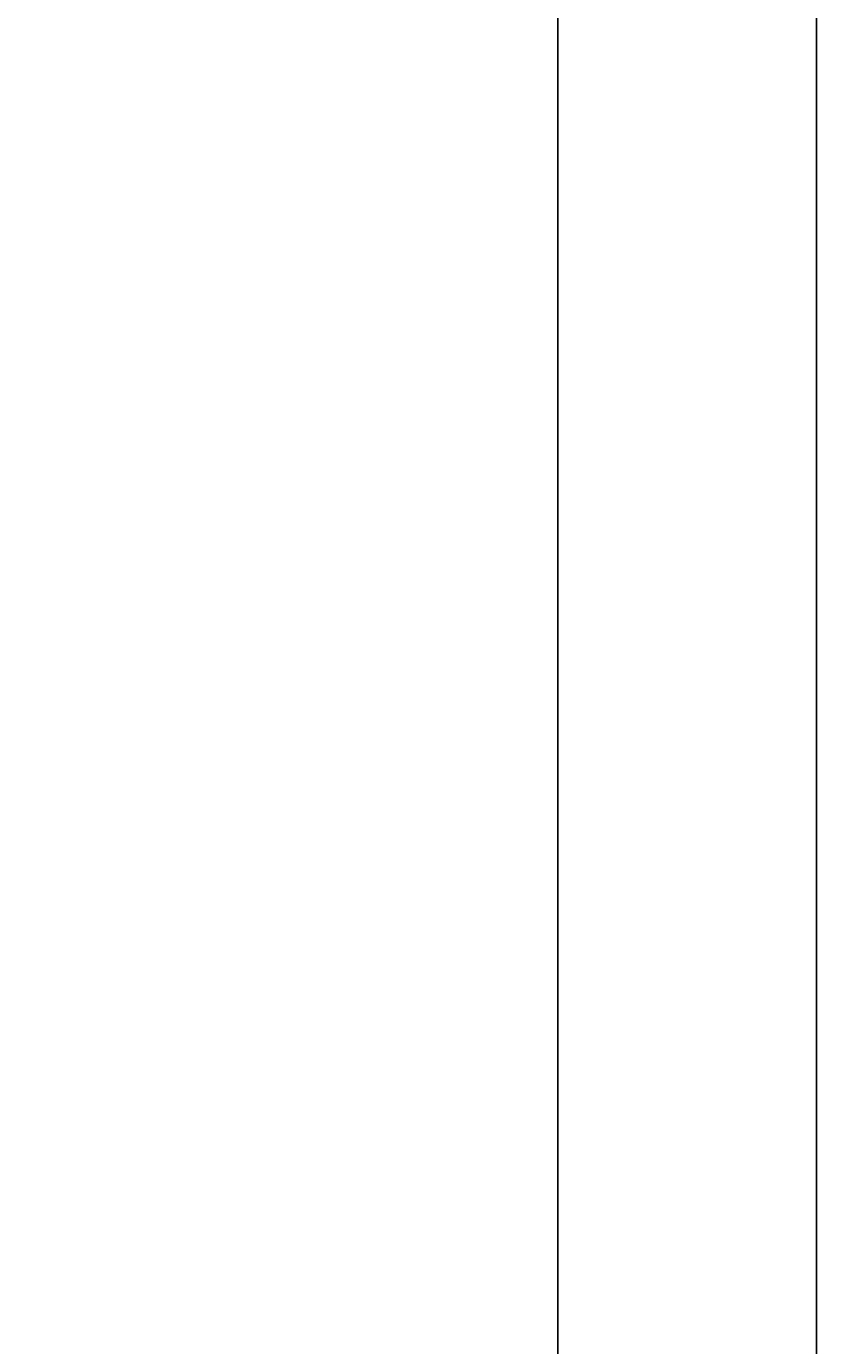
# Model space of a CAD drawing. Units: inches. Extents: x 1601 to 2297, y 1496 to 2631.
# Tile 23 of 57: x 2242 to 2297, y 1701 to 1793. Entities that reach past the tile are written whole.
import ezdxf

# ---------------------------------------------------------------- set-up
doc = ezdxf.new("R2010")
doc.units = ezdxf.units.IN
doc.layers.add('A-ANNO-DIMS', color=2, linetype='Continuous', lineweight=18)
doc.layers.add('A-ANNO-TTLB', color=7, linetype='Continuous', lineweight=25)
doc.styles.get("Standard").update_dxf_attribs({"font": 'arial.ttf'})
doc.dimstyles.get("Standard").update_dxf_attribs({"dimtxt": 0.18, "dimasz": 0.18, "dimexe": 0.18, "dimexo": 0.0625, "dimgap": 0.09, "dimtad": 0, "dimtih": 1, "dimtoh": 1, "dimdec": 4, "dimzin": 0, "dimdsep": 46, "dimtxsty": 'Standard', "dimcen": 0.09, "dimadec": 0, "dimazin": 0, "dimtfac": 1, "dimtdec": 4, "dimtofl": 0, "dimtmove": 0, "dimatfit": 3, "dimfxl": 1, "dimtolj": 1, "dimtzin": 0, "dimarcsym": 0})

# ---------------------------------------------------------------- blocks, each defined once
blk = doc.blocks.new('*D29')
at = {"layer": 'A-ANNO-DIMS', "color": 0, "lineweight": -2, "transparency": 16777216}
for p, q in [((2230.6, 2532.325), (2279.267, 2532.325)), ((2279.087, 2532.145), (2279.087, 2084.007)), ((2279.087, 1635.505), (2279.087, 2083.643)), ((2230.6, 1635.325), (2279.267, 1635.325))]:
    blk.add_line(p, q, dxfattribs=at)
at = {"layer": 'A-ANNO-DIMS', "color": 0, "transparency": 16777216}
for points in [[(2279.057, 2532.145), (2279.117, 2532.145), (2279.087, 2532.325)], [(2279.057, 1635.505), (2279.117, 1635.505), (2279.087, 1635.325)]]:
    blk.add_solid(points, dxfattribs=at)
at = {"layer": 'Defpoints', "color": 0, "transparency": 16777216}
for p in [(2230.537, 2532.325), (2279.087, 2532.325), (2230.537, 1635.325)]:
    blk.add_point(p, dxfattribs=at)
at = {"layer": 'A-ANNO-DIMS', "color": 0, "transparency": 16777216, "insert": (2279.087, 2083.825), "char_height": 0.18, "attachment_point": 5}
blk.add_mtext('\\A1;897', dxfattribs=at)

msp = doc.modelspace()

# ---------------------------------------------------------------- linework, layer by layer
at = {"layer": 'A-ANNO-TTLB'}
msp.add_lwpolyline([(1600.5933, 2631.1477), (2297.129, 2631.1477), (2297.129, 1496.1026), (1600.5933, 1496.1026)], close=True, dxfattribs=at)

# ---------------------------------------------------------------- dimensions: what is measured, and where the dimension line sits
at = {"layer": 'A-ANNO-DIMS'}
dim = msp.add_linear_dim(base=(2279.0873, 2532.3254), p1=(2230.5373, 1635.3254), p2=(2230.5373, 2532.3254), angle=90, dimstyle='Standard', override={"dimdec": 0, "dimlfac": 1, "dimrnd": 0, "dimzin": 0, "dimdsep": 46, "dimlunit": 2}, dxfattribs=at)
dim.commit()
dim.dimension.update_dxf_attribs({"geometry": '*D29', "text_midpoint": (2279.0873, 2083.8254)})

doc.saveas('drawing.dxf')
